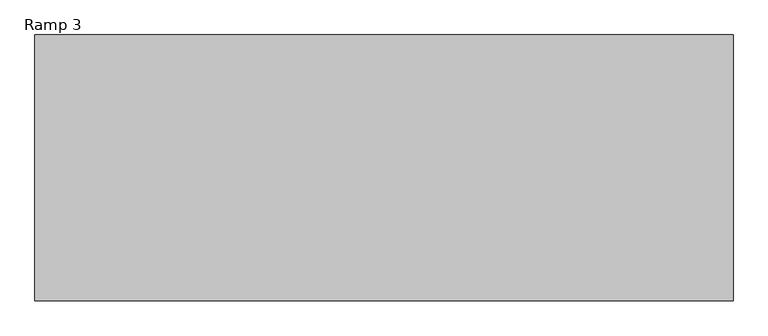
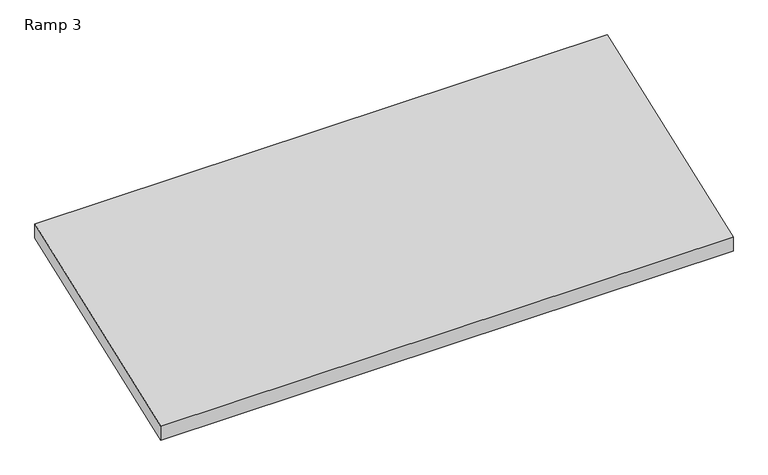
"""IFC4 building model written with IfcOpenShell, lengths in millimetres: ramp geometry, Ramp 3."""

from ifc_helpers import new_model, si_unit, frame, origin, place, context, project, spatial, polyline, outline, extrude, source, transform, mapped, element, save


def ramp_3_52017588(model_context):
    return source(origin(), model_context, "Body", "SweptSolid", [
        extrude(outline(polyline([(-13194.9643494, 0.0), (-11975.7643494, 457.2), (-11975.7643494, 375.8183643), (-13194.9643494, -81.3816357), (-13194.9643494, 0.0)])), frame((147.1271331, 0.0, 0.0), z_axis=(1.0, 0.0, 0.0), x_axis=(0.0, 1.0, 0.0)), (0.0, 0.0, 1.0), 3200.4),
    ])


if __name__ == "__main__":
    model = new_model("IFC4")
    model_context = context("Model", 3, world=origin())
    ifc_project = project(units=[si_unit("LENGTHUNIT", "METRE", prefix="MILLI")], contexts=[model_context])
    site = spatial("IfcSite", under=ifc_project)
    building = spatial("IfcBuilding", under=site)
    placement = place(None, origin())
    ramp_3_shape = ramp_3_52017588(model_context)
    element("IfcRamp", 1, ObjectType="Ramp 3", at=placement, inside=building, context=model_context, shape_type="MappedRepresentation", body=[
        mapped(ramp_3_shape, transform((0.0, 0.0, 0.0), x_axis=(1.0, 0.0, 0.0), y_axis=(0.0, 1.0, 0.0), z_axis=(0.0, 0.0, 1.0))),
    ])
    save(model, "model.ifc")

# Revit data of these elements
# Element 1 (IfcRamp, "Ramp 3")
#   Materials on its faces: "ramp"
# Materials
#   "ramp": class "Generic", colour RGB 123 104 76, transparency 0, Cost = 0
